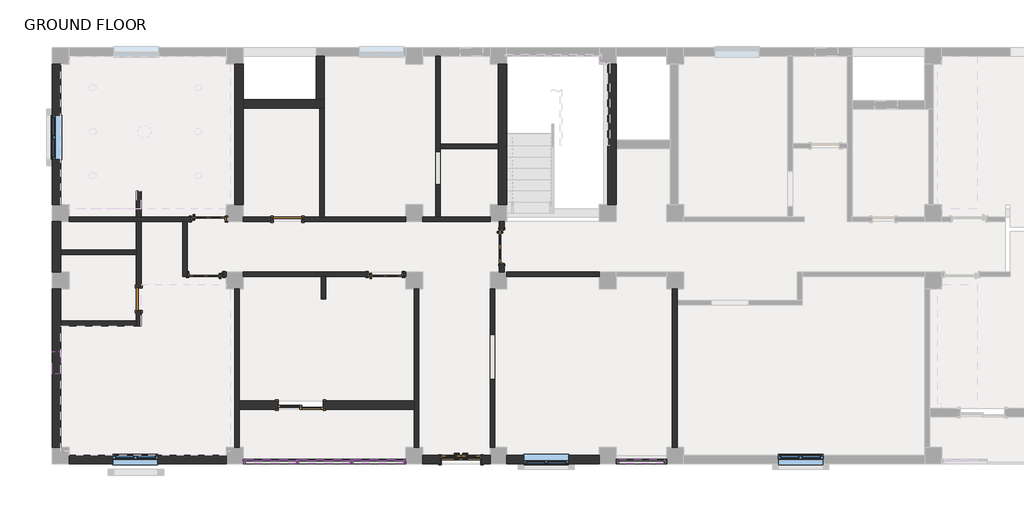
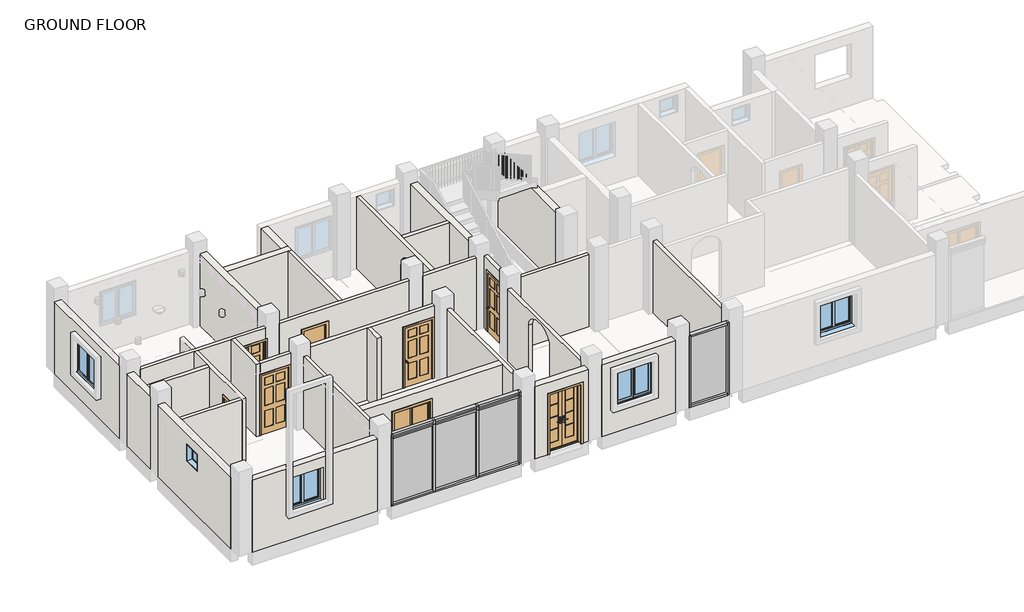
# One storey, part 1 of 5: 31 walls, 21 members, 8 doors, 7 plates, 5 windows.
# Revit data of these elements (continued)
# Element 71 (IfcWindow, "w2.0001 : 4' X 4' WINDOW") (continued)
#   Materials on its faces: "Fenster - Kunststoff", "Fenster - Kunststoff weiss", "Glass", "Fenster - Holz"
# Element 72 (IfcWindow, "w2.0001 : 4' X 4' WINDOW")
#   Mark = "94"
#   Einbautiefe (von außen) = 0' - 5.51181"
#   Kippflügel = yes
#   Drehflügel im Grundriß darstellen = no
#   Drehflügel = yes
#   Rahmen = none
#   Glas = none
#   Flügel = none
#   Fensterbank innen = none
#   Fensterbank aussen = none
#   Phase Created = New Construction
#   Materials on its faces: "Fenster - Kunststoff", "Fenster - Kunststoff weiss", "Glass", "Fenster - Holz"
# Materials
#   "Glass": class "Glass", colour RGB 0 128 192, transparency 0.75, Description = "Soda Lime Glass", Cost = 0
#   "Wood - Birch - Solid Stained Light Low Gloss": class "Wood", colour RGB 210 159 95, transparency 0, Cost = 0
#   "Paint - Sienna": colour RGB 118 70 51, transparency 0, Cost = 0
#   "Cherry": class "Wood", colour RGB 226 177 128, transparency 0, Description = "Prunus Serotina", Cost = 0
#   "Aluminum": class "Metal", colour RGB 247 247 247, transparency 0, Description = "Aluminum 6061", Cost = 0
#   "Door - Panel": class "Wood", colour RGB 210 159 95, transparency 0, Cost = 0
#   "Door - Frame": colour RGB 118 70 51, transparency 0, Cost = 0
#   "SAND BEIGE PAINT": class "Generic", colour RGB 120 120 120, transparency 0, Cost = 0
#   "Sash": class "Wood", colour RGB 224 178 126, transparency 0, Cost = 0
#   "WINDOW FRAMING": class "Generic", colour RGB 120 120 120, transparency 0, Cost = 0
#   "Fenster - Kunststoff": colour RGB 249 249 249, transparency 0
#   "Fenster - Kunststoff weiss": colour RGB 249 249 249, transparency 0
#   "Fenster - Holz": colour RGB 216 135 75, transparency 0
# Room at (5469.642, -1195.829) mm, phase "New Construction", upper level "GROUND FLOOR", upper offset 10' - 0", lower offset 0' - 0"
#   Number = "1"
#   Name = "Room"
# Room at (5469.642, -3469.129) mm, phase "New Construction", upper level "GROUND FLOOR", upper offset 10' - 0", lower offset 0' - 0"
#   Number = "2"
#   Name = "Room"
# Room at (-4020.146, -1202.179) mm, phase "New Construction", upper level "GROUND FLOOR", upper offset 10' - 0", lower offset 0' - 0"
#   Number = "3"
#   Name = "UTILITY"
# Room at (669.042, -1176.779) mm, phase "New Construction", upper level "GROUND FLOOR", upper offset 10' - 0", lower offset 0' - 0"
#   Number = "4"
#   Name = "lift"
# Room at (10654.013, -10360.818) mm, phase "New Construction", upper level "GROUND FLOOR", upper offset 10' - 0", lower offset 0' - 0"
#   Number = "5"
#   Name = "VERANDA"
# Room at (-4451.946, -8864.424) mm, phase "New Construction", upper level "GROUND FLOOR", upper offset 10' - 0", lower offset 0' - 0"
#   Number = "6"
#   Name = "Room"
# Room at (-7919.046, -10322.718) mm, phase "New Construction", upper level "GROUND FLOOR", upper offset 10' - 0", lower offset 0' - 0"
#   Number = "7"
#   Name = "VERANDA"
# Room at (-14141.443, -6333.723) mm, phase "New Construction", upper level "GROUND FLOOR", upper offset 10' - 0", lower offset 0' - 0"
#   Number = "8"
#   Name = "TOILET"
# Room at (-14141.443, -4916.929) mm, phase "New Construction", upper level "GROUND FLOOR", upper offset 10' - 0", lower offset 0' - 0"
#   Number = "9"
#   Name = "Room"
# Room at (-9176.346, -2897.629) mm, phase "New Construction", upper level "GROUND FLOOR", upper offset 10' - 0", lower offset 0' - 0"
#   Number = "10"
#   Name = "TOILET"
# Room at (-12783.146, -2192.779) mm, phase "New Construction", upper level "GROUND FLOOR", upper offset 10' - 0", lower offset 0' - 0"
#   Number = "11"
#   Name = "BED ROOM"
# Room at (-6496.646, -2192.779) mm, phase "New Construction", upper level "GROUND FLOOR", upper offset 10' - 0", lower offset 0' - 0"
#   Number = "12"
#   Name = "KITCHEN"
# Room, not placed, phase "New Construction", upper offset 0' - 0", lower offset 0' - 0"
#   Number = "13"
#   Name = "Room"
# Room, not placed, phase "New Construction", upper offset 0' - 0", lower offset 0' - 0"
#   Number = "14"
#   Name = "Room"
# Room at (10679.413, -2332.479) mm, phase "New Construction", upper level "GROUND FLOOR", upper offset 10' - 0", lower offset 0' - 0"
#   Number = "15"
#   Name = "BED ROOM 6"
# Room at (7379.202, -2916.679) mm, phase "New Construction", upper level "GROUND FLOOR", upper offset 10' - 0", lower offset 0' - 0"
#   Number = "16"
#   Name = "Room"
# Room, not placed, phase "New Construction", upper offset 0' - 0", lower offset 0' - 0"
#   Number = "17"
#   Name = "DINING ROOM"
# Room at (10654.013, -7232.474) mm, phase "New Construction", upper level "GROUND FLOOR", upper offset 10' - 0", lower offset 0' - 0"
#   Number = "18"
#   Name = "BED ROOM 3"
# Room, not placed, phase "New Construction", upper offset 0' - 0", lower offset 0' - 0"
#   Number = "19"
#   Name = "STAIRS"
# Room, not placed, phase "New Construction", upper offset 0' - 0", lower offset 0' - 0"
#   Number = "20"
#   Name = "LIVING ROOM"
# Room, not placed, phase "New Construction", upper offset 0' - 0", lower offset 0' - 0"
#   Number = "21"
#   Name = "PASSAGE"
# Room at (-12808.546, -7734.124) mm, phase "New Construction", upper level "GROUND FLOOR", upper offset 10' - 0", lower offset 0' - 0"
#   Number = "22"
#   Name = "BED ROOM 2"
# Room at (-7919.046, -7740.474) mm, phase "New Construction", upper level "GROUND FLOOR", upper offset 10' - 0", lower offset 0' - 0"
#   Number = "23"
#   Name = "Room"
